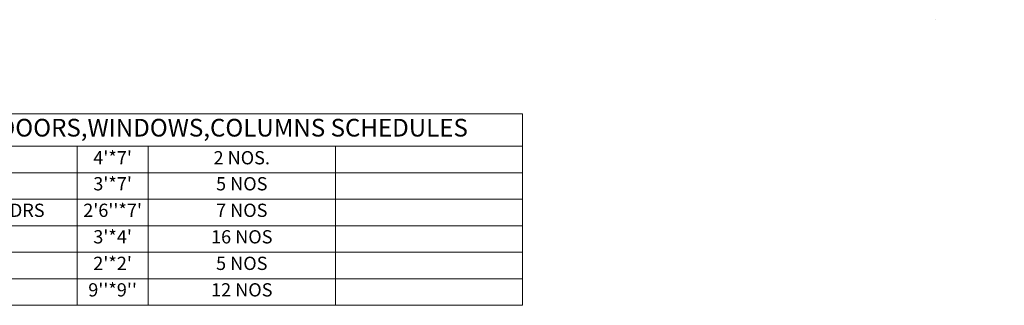
# Model space of a CAD drawing. Units: inches. Extents: x 20414 to 21627, y 49019 to 50314.
# Tile 10 of 10: x 21087 to 21627, y 49803 to 49960. Entities that reach past the tile are written whole.
import ezdxf

# ---------------------------------------------------------------- set-up
doc = ezdxf.new("R2010")
doc.units = ezdxf.units.IN
for name, color, linetype, lineweight in [('A-ANNO-SCHD', 7, 'Continuous', 18), ('A-FLOR-STRS-PATT', 4, 'Continuous', 13), ('A-REF', 8, 'Continuous', 13)]:
    doc.layers.add(name, color=color, linetype=linetype, lineweight=lineweight)
doc.styles.get("Standard").update_dxf_attribs({"font": 'arial.ttf'})

# ---------------------------------------------------------------- blocks, each defined once
blk = doc.blocks.new('*T57')
at = {"layer": 'A-ANNO-SCHD', "transparency": 16777216}
for p, q in [((0, 0), (411.04, 0)), ((0, 0), (0, -105.19)), ((411.04, 0), (411.04, -105.19)), ((0, -17.8), (411.04, -17.8)), ((166.47, -17.8), (166.47, -105.19)), ((205.52, -17.8), (205.52, -105.19)), ((308.28, -17.8), (308.28, -105.19)), ((0, -32.37), (411.04, -32.37)), ((0, -46.93), (411.04, -46.93)), ((0, -61.49), (411.04, -61.49)), ((0, -76.06), (411.04, -76.06)), ((0, -90.62), (411.04, -90.62)), ((0, -105.19), (411.04, -105.19))]:
    blk.add_line(p, q, dxfattribs=at)
at = {"layer": 'A-ANNO-SCHD', "color": 0, "transparency": 16777216}
for s, insert, char_height, width, attachment_point in [('GF,1ST FLOOR-DOORS,WINDOWS,COLUMNS SCHEDULES', (205.52, -8.9), 9.7096, 406.1845, 5), ('MAIN DOOR', (83.23, -25.08), 7.282, 161.6127, 5), ("4'*7'", (185.99, -25.08), 7.282, 34.1974, 5), ('2 NOS.', (256.9, -25.08), 7.282, 97.905, 5), ('BED ROOM DOOR', (83.23, -34.79), 7.2822, 161.6127, 2), ("3'*7'", (185.99, -34.79), 7.282, 34.1974, 2), ('5 NOS', (256.9, -34.79), 7.282, 97.905, 2), ('TOILET, BALCONY PUJA DRS', (83.23, -49.36), 7.2822, 161.6127, 2), ("2'6''*7'", (185.99, -49.36), 7.282, 34.1974, 2), ('7 NOS', (256.9, -49.36), 7.282, 97.905, 2), ('WINDOWS', (83.23, -63.92), 7.282, 161.6127, 2), ("3'*4'", (185.99, -63.92), 7.282, 34.1974, 2), ('16 NOS', (256.9, -63.92), 7.282, 97.905, 2), ('VENTILATORS', (83.23, -78.49), 7.2822, 161.6127, 2), ("2'*2'", (185.99, -78.49), 7.282, 34.1974, 2), ('5 NOS', (256.9, -78.49), 7.282, 97.905, 2), ('COLUMNS', (83.23, -93.05), 7.282, 161.6127, 2), ("9''*9''", (185.99, -93.05), 7.282, 34.1974, 2), ('12 NOS', (256.9, -93.05), 7.282, 97.905, 2)]:
    blk.add_mtext(s, dxfattribs=dict(at, insert=insert, char_height=char_height, width=width, attachment_point=attachment_point))

msp = doc.modelspace()

# ---------------------------------------------------------------- hatches: boundary and pattern name
at = {"layer": 'A-FLOR-STRS-PATT'}
h = msp.add_hatch(dxfattribs=at)
h.set_pattern_fill('AR-RROOF', color=256)
h.set_pattern_definition([(0, (-53781.747, -25819.044), (55.88, 25.4), [381, -50.8, 127, -25.4]), (0, (-53747.965, -25806.344), (-25.4, 33.782), [76.2, -8.382, 152.4, -19.05]), (0, (-53769.047, -25797.454), (132.08, 17.018), [203.2, -35.56, 101.6, -25.4])])
h.paths.add_polyline_path([(21625.06, 49959.02), (21622.3, 49954.62), (21625.06, 49954.62)])
h.paths.add_polyline_path([(21625.06, 49959.02), (21625.06, 49954.62), (21627.4, 49954.62)])

# ---------------------------------------------------------------- linework, layer by layer
at = {"layer": 'A-REF'}
msp.add_lwpolyline([(21589.7, 49960.35), (21589.7, 49960.35)], close=True, dxfattribs=at)

# ---------------------------------------------------------------- block references
msp.add_blockref('*T57', (20951.88, 49908.67))

doc.saveas('drawing.dxf')
